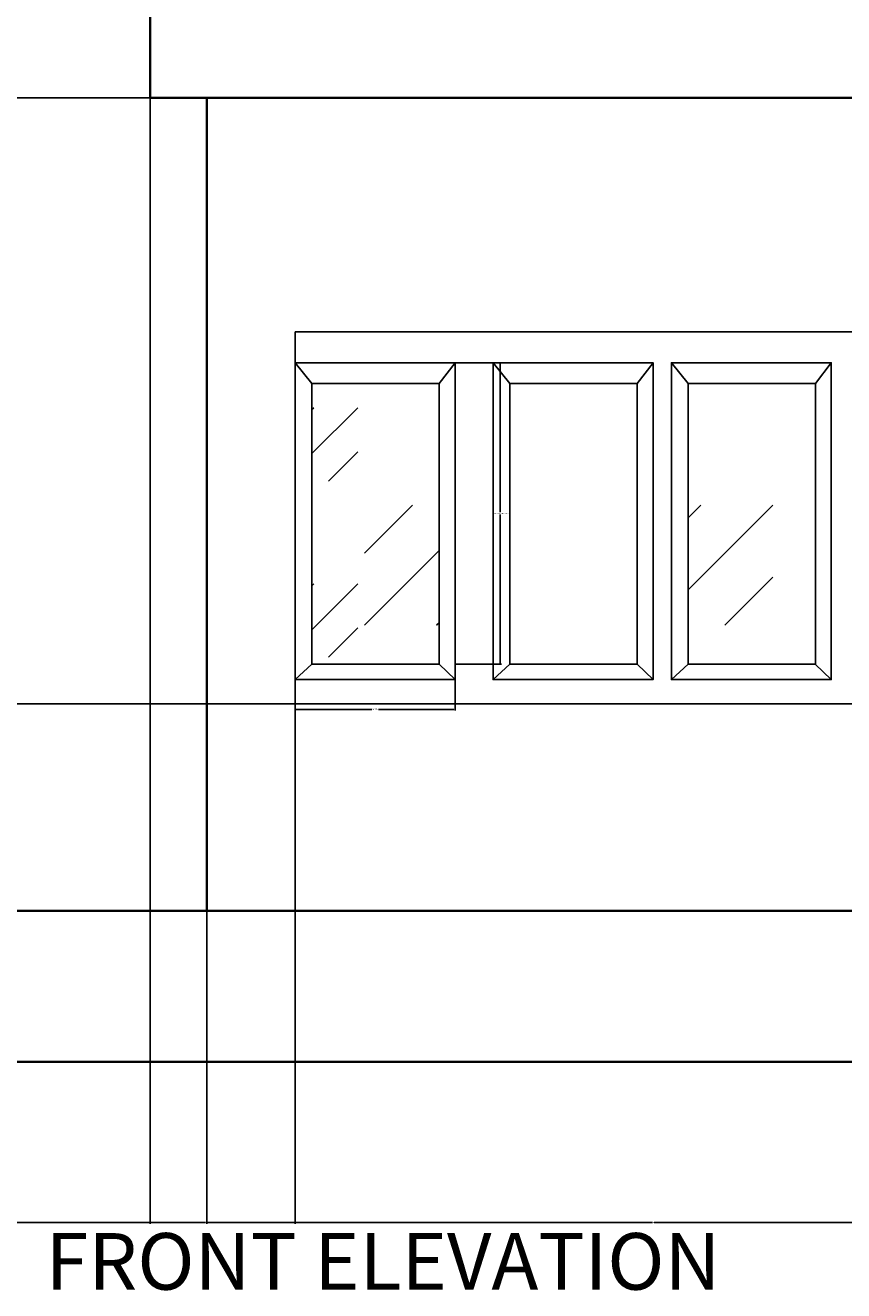
# Model space of a CAD drawing. Units: inches. Extents: x 93 to 565, y 123 to 656.
# Tile 2 of 18: x 267 to 397, y 123 to 324. Entities that reach past the tile are written whole.
import ezdxf

# ---------------------------------------------------------------- set-up
doc = ezdxf.new("R2010")
doc.units = ezdxf.units.IN
doc.header["$MEASUREMENT"] = 0
for name, color, linetype, lineweight in [('A-ANNO-DIMS', 2, 'Continuous', 18), ('A-ANNO-TEXT', 7, 'Continuous', 25), ('A-ELEV', 7, 'Continuous', 35), ('A-GLAZ', 4, 'Continuous', 25)]:
    doc.layers.add(name, color=color, linetype=linetype, lineweight=lineweight)
doc.styles.get("Standard").update_dxf_attribs({"font": 'arial.ttf'})
doc.dimstyles.get("Standard").update_dxf_attribs({"dimtxt": 0.18, "dimasz": 0.18, "dimexe": 0.18, "dimexo": 0.0625, "dimgap": 0.09, "dimtad": 0, "dimtih": 1, "dimtoh": 1, "dimdec": 4, "dimzin": 0, "dimdsep": 46, "dimtxsty": 'Standard', "dimcen": 0.09, "dimadec": 0, "dimazin": 0, "dimtfac": 1, "dimtdec": 4, "dimtofl": 0, "dimtmove": 0, "dimatfit": 3, "dimfxl": 1, "dimtolj": 1, "dimtzin": 0, "dimarcsym": 0})

# ---------------------------------------------------------------- blocks, each defined once
blk = doc.blocks.new('WIN-CASEMENT-LARGE')
blk.add_lwpolyline([(2.67, 44.6), (0, 47.91), (25.42, 47.91), (22.89, 44.6)])
blk.add_lwpolyline([(2.67, 44.6), (22.89, 44.6), (22.89, 0), (2.67, 0)], close=True)
blk = doc.blocks.new('*D18')
at = {"layer": 'A-ANNO-DIMS', "color": 0, "lineweight": -2, "transparency": 16777216}
for p, q in [((335.22, 270.85), (342.53, 270.85)), ((342.35, 270.67), (342.35, 247.08)), ((342.35, 223.12), (342.35, 246.71)), ((335.22, 222.94), (342.53, 222.94))]:
    blk.add_line(p, q, dxfattribs=at)
at = {"layer": 'A-ANNO-DIMS', "color": 0, "transparency": 16777216}
for points in [[(342.32, 270.67), (342.38, 270.67), (342.35, 270.85)], [(342.32, 223.12), (342.38, 223.12), (342.35, 222.94)]]:
    blk.add_solid(points, dxfattribs=at)
at = {"layer": 'Defpoints', "color": 0, "transparency": 16777216}
for p in [(335.16, 270.85), (342.35, 270.85), (335.16, 222.94)]:
    blk.add_point(p, dxfattribs=at)
at = {"layer": 'A-ANNO-DIMS', "color": 0, "transparency": 16777216, "insert": (342.35, 246.89), "char_height": 0.18, "attachment_point": 5}
blk.add_mtext('\\A1;LARGE WINDOW 48 TYP.', dxfattribs=at)
blk = doc.blocks.new('*D19')
at = {"layer": 'A-ANNO-DIMS', "color": 0, "lineweight": -2, "transparency": 16777216}
for p, q in [((309.74, 222.88), (309.74, 215.57)), ((335.16, 222.88), (335.16, 215.57)), ((309.92, 215.75), (321.92, 215.75)), ((334.98, 215.75), (322.98, 215.75))]:
    blk.add_line(p, q, dxfattribs=at)
at = {"layer": 'A-ANNO-DIMS', "color": 0, "transparency": 16777216}
for points in [[(309.92, 215.78), (309.92, 215.72), (309.74, 215.75)], [(334.98, 215.78), (334.98, 215.72), (335.16, 215.75)]]:
    blk.add_solid(points, dxfattribs=at)
at = {"layer": 'Defpoints', "color": 0, "transparency": 16777216}
for p in [(309.74, 222.94), (335.16, 222.94), (335.16, 215.75)]:
    blk.add_point(p, dxfattribs=at)
at = {"layer": 'A-ANNO-DIMS', "color": 0, "transparency": 16777216, "insert": (322.45, 215.75), "char_height": 0.18, "attachment_point": 5}
blk.add_mtext('\\A1;25 TYP.', dxfattribs=at)
blk = doc.blocks.new('*D28')
at = {"layer": 'A-ANNO-DIMS', "color": 0, "lineweight": -2, "transparency": 16777216}
for p, q in [((210.54, 519.04), (210.54, 134)), ((295.69, 183.67), (295.69, 134)), ((210.72, 134.18), (252.72, 134.18)), ((295.51, 134.18), (253.51, 134.18))]:
    blk.add_line(p, q, dxfattribs=at)
at = {"layer": 'A-ANNO-DIMS', "color": 0, "transparency": 16777216}
for points in [[(210.72, 134.21), (210.72, 134.15), (210.54, 134.18)], [(295.51, 134.21), (295.51, 134.15), (295.69, 134.18)]]:
    blk.add_solid(points, dxfattribs=at)
at = {"layer": 'Defpoints', "color": 0, "transparency": 16777216}
for p in [(210.54, 519.1), (295.69, 183.73), (295.69, 134.18)]:
    blk.add_point(p, dxfattribs=at)
at = {"layer": 'A-ANNO-DIMS', "color": 0, "transparency": 16777216, "insert": (253.12, 134.18), "char_height": 0.18, "attachment_point": 5}
blk.add_mtext('\\A1;85.14', dxfattribs=at)
blk = doc.blocks.new('*D29')
at = {"layer": 'A-ANNO-DIMS', "color": 0, "lineweight": -2, "transparency": 16777216}
for p, q in [((437.19, 594.34), (437.19, 134)), ((295.69, 183.67), (295.69, 134)), ((295.87, 134.18), (366.05, 134.18)), ((437.01, 134.18), (366.82, 134.18))]:
    blk.add_line(p, q, dxfattribs=at)
at = {"layer": 'A-ANNO-DIMS', "color": 0, "transparency": 16777216}
for points in [[(295.87, 134.21), (295.87, 134.15), (295.69, 134.18)], [(437.01, 134.21), (437.01, 134.15), (437.19, 134.18)]]:
    blk.add_solid(points, dxfattribs=at)
at = {"layer": 'Defpoints', "color": 0, "transparency": 16777216}
for p in [(437.19, 594.4), (295.69, 183.73), (437.19, 134.18)]:
    blk.add_point(p, dxfattribs=at)
at = {"layer": 'A-ANNO-DIMS', "color": 0, "transparency": 16777216, "insert": (366.44, 134.18), "char_height": 0.18, "attachment_point": 5}
blk.add_mtext('\\A1;141.5', dxfattribs=at)
blk = doc.blocks.new('*D31')
at = {"layer": 'A-ANNO-DIMS', "color": 0, "lineweight": -2, "transparency": 16777216}
for p, q in [((417.87, 630.4), (564.81, 630.4)), ((564.63, 630.22), (564.63, 395.25)), ((564.63, 159.91), (564.63, 394.89)), ((119.14, 159.73), (564.81, 159.73))]:
    blk.add_line(p, q, dxfattribs=at)
at = {"layer": 'A-ANNO-DIMS', "color": 0, "transparency": 16777216}
for points in [[(564.6, 630.22), (564.66, 630.22), (564.63, 630.4)], [(564.6, 159.91), (564.66, 159.91), (564.63, 159.73)]]:
    blk.add_solid(points, dxfattribs=at)
at = {"layer": 'Defpoints', "color": 0, "transparency": 16777216}
for p in [(417.81, 630.4), (564.63, 630.4), (119.08, 159.73)]:
    blk.add_point(p, dxfattribs=at)
at = {"layer": 'A-ANNO-DIMS', "color": 0, "transparency": 16777216, "insert": (564.63, 395.07), "char_height": 0.18, "attachment_point": 5}
blk.add_mtext('\\A1;470.7', dxfattribs=at)
blk = doc.blocks.new('*D33')
at = {"layer": 'A-ANNO-DIMS', "color": 0, "lineweight": -2, "transparency": 16777216}
for p, q in [((286.62, 312.95), (93.35, 312.95)), ((93.53, 312.77), (93.53, 248.52)), ((93.53, 183.91), (93.53, 248.16)), ((119.02, 183.73), (93.35, 183.73))]:
    blk.add_line(p, q, dxfattribs=at)
at = {"layer": 'A-ANNO-DIMS', "color": 0, "transparency": 16777216}
for points in [[(93.5, 312.77), (93.56, 312.77), (93.53, 312.95)], [(93.5, 183.91), (93.56, 183.91), (93.53, 183.73)]]:
    blk.add_solid(points, dxfattribs=at)
at = {"layer": 'Defpoints', "color": 0, "transparency": 16777216}
for p in [(93.53, 312.95), (286.69, 312.95), (119.08, 183.73)]:
    blk.add_point(p, dxfattribs=at)
at = {"layer": 'A-ANNO-DIMS', "color": 0, "transparency": 16777216, "insert": (93.53, 248.34), "char_height": 0.18, "attachment_point": 5}
blk.add_mtext('\\A1;129.22', dxfattribs=at)
blk = doc.blocks.new('*D34')
at = {"layer": 'A-ANNO-DIMS', "color": 0, "lineweight": -2, "transparency": 16777216}
for p, q in [((286.62, 363.73), (93.35, 363.73)), ((93.53, 363.55), (93.53, 338.52)), ((93.53, 313.13), (93.53, 338.16)), ((286.62, 312.95), (93.35, 312.95))]:
    blk.add_line(p, q, dxfattribs=at)
at = {"layer": 'A-ANNO-DIMS', "color": 0, "transparency": 16777216}
for points in [[(93.5, 363.55), (93.56, 363.55), (93.53, 363.73)], [(93.5, 313.13), (93.56, 313.13), (93.53, 312.95)]]:
    blk.add_solid(points, dxfattribs=at)
at = {"layer": 'Defpoints', "color": 0, "transparency": 16777216}
for p in [(93.53, 363.73), (286.69, 363.73), (286.69, 312.95)]:
    blk.add_point(p, dxfattribs=at)
at = {"layer": 'A-ANNO-DIMS', "color": 0, "transparency": 16777216, "insert": (93.53, 338.34), "char_height": 0.18, "attachment_point": 5}
blk.add_mtext('\\A1;50.78', dxfattribs=at)
blk = doc.blocks.new('*D51')
at = {"layer": 'A-ANNO-DIMS', "color": 0, "lineweight": -2, "transparency": 16777216}
for p, q in [((286.69, 312.89), (286.69, 134)), ((295.69, 312.89), (295.69, 134)), ((286.87, 134.18), (291.04, 134.18)), ((295.51, 134.18), (291.34, 134.18))]:
    blk.add_line(p, q, dxfattribs=at)
at = {"layer": 'A-ANNO-DIMS', "color": 0, "transparency": 16777216}
for points in [[(286.87, 134.21), (286.87, 134.15), (286.69, 134.18)], [(295.51, 134.21), (295.51, 134.15), (295.69, 134.18)]]:
    blk.add_solid(points, dxfattribs=at)
at = {"layer": 'Defpoints', "color": 0, "transparency": 16777216}
for p in [(286.69, 312.95), (295.69, 312.95), (295.69, 134.18)]:
    blk.add_point(p, dxfattribs=at)
at = {"layer": 'A-ANNO-DIMS', "color": 0, "transparency": 16777216, "insert": (291.19, 134.18), "char_height": 0.18, "attachment_point": 5}
blk.add_mtext('\\A1;9', dxfattribs=at)
blk = doc.blocks.new('*D55')
at = {"layer": 'A-ANNO-DIMS', "color": 0, "lineweight": -2, "transparency": 16777216}
for p, q in [((309.74, 216.57), (309.74, 134)), ((295.69, 183.67), (295.69, 134)), ((295.87, 134.18), (302.26, 134.18)), ((309.56, 134.18), (303.17, 134.18))]:
    blk.add_line(p, q, dxfattribs=at)
at = {"layer": 'A-ANNO-DIMS', "color": 0, "transparency": 16777216}
for points in [[(295.87, 134.21), (295.87, 134.15), (295.69, 134.18)], [(309.56, 134.21), (309.56, 134.15), (309.74, 134.18)]]:
    blk.add_solid(points, dxfattribs=at)
at = {"layer": 'Defpoints', "color": 0, "transparency": 16777216}
for p in [(309.74, 216.63), (295.69, 183.73), (309.74, 134.18)]:
    blk.add_point(p, dxfattribs=at)
at = {"layer": 'A-ANNO-DIMS', "color": 0, "transparency": 16777216, "insert": (302.72, 134.18), "char_height": 0.18, "attachment_point": 5}
blk.add_mtext('\\A1;14.056', dxfattribs=at)
blk = doc.blocks.new('*D56')
at = {"layer": 'A-ANNO-DIMS', "color": 0, "lineweight": -2, "transparency": 16777216}
for p, q in [((309.74, 275.71), (309.74, 134)), ((424.3, 275.71), (424.3, 134)), ((309.92, 134.18), (366.57, 134.18)), ((424.12, 134.18), (367.48, 134.18))]:
    blk.add_line(p, q, dxfattribs=at)
at = {"layer": 'A-ANNO-DIMS', "color": 0, "transparency": 16777216}
for points in [[(309.92, 134.21), (309.92, 134.15), (309.74, 134.18)], [(424.12, 134.21), (424.12, 134.15), (424.3, 134.18)]]:
    blk.add_solid(points, dxfattribs=at)
at = {"layer": 'Defpoints', "color": 0, "transparency": 16777216}
for p in [(309.74, 275.77), (424.3, 275.77), (424.3, 134.18)]:
    blk.add_point(p, dxfattribs=at)
at = {"layer": 'A-ANNO-DIMS', "color": 0, "transparency": 16777216, "insert": (367.02, 134.18), "char_height": 0.18, "attachment_point": 5}
blk.add_mtext('\\A1;114.56', dxfattribs=at)
blk = doc.blocks.new('*D58')
at = {"layer": 'A-ANNO-DIMS', "color": 0, "lineweight": -2, "transparency": 16777216}
for p, q in [((309.68, 216.63), (93.35, 216.63)), ((93.53, 216.45), (93.53, 200.36)), ((93.53, 183.91), (93.53, 200)), ((295.62, 183.73), (93.35, 183.73))]:
    blk.add_line(p, q, dxfattribs=at)
at = {"layer": 'A-ANNO-DIMS', "color": 0, "transparency": 16777216}
for points in [[(93.5, 216.45), (93.56, 216.45), (93.53, 216.63)], [(93.5, 183.91), (93.56, 183.91), (93.53, 183.73)]]:
    blk.add_solid(points, dxfattribs=at)
at = {"layer": 'Defpoints', "color": 0, "transparency": 16777216}
for p in [(309.74, 216.63), (93.53, 183.73), (295.69, 183.73)]:
    blk.add_point(p, dxfattribs=at)
at = {"layer": 'A-ANNO-DIMS', "color": 0, "transparency": 16777216, "insert": (93.53, 200.18), "char_height": 0.18, "attachment_point": 5}
blk.add_mtext('\\A1;32.9', dxfattribs=at)
blk = doc.blocks.new('*D107')
at = {"layer": 'A-ANNO-DIMS', "color": 0, "lineweight": -2, "transparency": 16777216}
for p, q in [((210.54, 519.04), (210.54, 134)), ((295.69, 183.67), (295.69, 134)), ((210.72, 134.18), (252.65, 134.18)), ((295.51, 134.18), (253.58, 134.18))]:
    blk.add_line(p, q, dxfattribs=at)
at = {"layer": 'A-ANNO-DIMS', "color": 0, "transparency": 16777216}
for points in [[(210.72, 134.21), (210.72, 134.15), (210.54, 134.18)], [(295.51, 134.21), (295.51, 134.15), (295.69, 134.18)]]:
    blk.add_solid(points, dxfattribs=at)
at = {"layer": 'Defpoints', "color": 0, "transparency": 16777216}
for p in [(210.54, 519.1), (295.69, 183.73), (295.69, 134.18)]:
    blk.add_point(p, dxfattribs=at)
at = {"layer": 'A-ANNO-DIMS', "color": 0, "transparency": 16777216, "insert": (253.12, 134.18), "char_height": 0.18, "attachment_point": 5}
blk.add_mtext('\\A1;85.143', dxfattribs=at)
blk = doc.blocks.new('*D108')
at = {"layer": 'A-ANNO-DIMS', "color": 0, "lineweight": -2, "transparency": 16777216}
for p, q in [((437.19, 594.34), (437.19, 134)), ((295.69, 183.67), (295.69, 134)), ((295.87, 134.18), (365.93, 134.18)), ((437.01, 134.18), (366.95, 134.18))]:
    blk.add_line(p, q, dxfattribs=at)
at = {"layer": 'A-ANNO-DIMS', "color": 0, "transparency": 16777216}
for points in [[(295.87, 134.21), (295.87, 134.15), (295.69, 134.18)], [(437.01, 134.21), (437.01, 134.15), (437.19, 134.18)]]:
    blk.add_solid(points, dxfattribs=at)
at = {"layer": 'Defpoints', "color": 0, "transparency": 16777216}
for p in [(437.19, 594.4), (295.69, 183.73), (437.19, 134.18)]:
    blk.add_point(p, dxfattribs=at)
at = {"layer": 'A-ANNO-DIMS', "color": 0, "transparency": 16777216, "insert": (366.44, 134.18), "char_height": 0.18, "attachment_point": 5}
blk.add_mtext('\\A1;141.501', dxfattribs=at)
blk = doc.blocks.new('*D110')
at = {"layer": 'A-ANNO-DIMS', "color": 0, "lineweight": -2, "transparency": 16777216}
for p, q in [((417.87, 630.4), (564.81, 630.4)), ((564.63, 630.22), (564.63, 395.25)), ((564.63, 159.91), (564.63, 394.89)), ((119.14, 159.73), (564.81, 159.73))]:
    blk.add_line(p, q, dxfattribs=at)
at = {"layer": 'A-ANNO-DIMS', "color": 0, "transparency": 16777216}
for points in [[(564.6, 630.22), (564.66, 630.22), (564.63, 630.4)], [(564.6, 159.91), (564.66, 159.91), (564.63, 159.73)]]:
    blk.add_solid(points, dxfattribs=at)
at = {"layer": 'Defpoints', "color": 0, "transparency": 16777216}
for p in [(417.81, 630.4), (564.63, 630.4), (119.08, 159.73)]:
    blk.add_point(p, dxfattribs=at)
at = {"layer": 'A-ANNO-DIMS', "color": 0, "transparency": 16777216, "insert": (564.63, 395.07), "char_height": 0.18, "attachment_point": 5}
blk.add_mtext('\\A1;470.673', dxfattribs=at)
blk = doc.blocks.new('*D112')
at = {"layer": 'A-ANNO-DIMS', "color": 0, "lineweight": -2, "transparency": 16777216}
for p, q in [((286.62, 312.95), (93.35, 312.95)), ((93.53, 312.77), (93.53, 248.52)), ((93.53, 183.91), (93.53, 248.16)), ((119.02, 183.73), (93.35, 183.73))]:
    blk.add_line(p, q, dxfattribs=at)
at = {"layer": 'A-ANNO-DIMS', "color": 0, "transparency": 16777216}
for points in [[(93.5, 312.77), (93.56, 312.77), (93.53, 312.95)], [(93.5, 183.91), (93.56, 183.91), (93.53, 183.73)]]:
    blk.add_solid(points, dxfattribs=at)
at = {"layer": 'Defpoints', "color": 0, "transparency": 16777216}
for p in [(93.53, 312.95), (286.69, 312.95), (119.08, 183.73)]:
    blk.add_point(p, dxfattribs=at)
at = {"layer": 'A-ANNO-DIMS', "color": 0, "transparency": 16777216, "insert": (93.53, 248.34), "char_height": 0.18, "attachment_point": 5}
blk.add_mtext('\\A1;129.217', dxfattribs=at)
blk = doc.blocks.new('*D113')
at = {"layer": 'A-ANNO-DIMS', "color": 0, "lineweight": -2, "transparency": 16777216}
for p, q in [((286.62, 363.73), (93.35, 363.73)), ((93.53, 363.55), (93.53, 338.52)), ((93.53, 313.13), (93.53, 338.16)), ((286.62, 312.95), (93.35, 312.95))]:
    blk.add_line(p, q, dxfattribs=at)
at = {"layer": 'A-ANNO-DIMS', "color": 0, "transparency": 16777216}
for points in [[(93.5, 363.55), (93.56, 363.55), (93.53, 363.73)], [(93.5, 313.13), (93.56, 313.13), (93.53, 312.95)]]:
    blk.add_solid(points, dxfattribs=at)
at = {"layer": 'Defpoints', "color": 0, "transparency": 16777216}
for p in [(93.53, 363.73), (286.69, 363.73), (286.69, 312.95)]:
    blk.add_point(p, dxfattribs=at)
at = {"layer": 'A-ANNO-DIMS', "color": 0, "transparency": 16777216, "insert": (93.53, 338.34), "char_height": 0.18, "attachment_point": 5}
blk.add_mtext('\\A1;50.783', dxfattribs=at)
blk = doc.blocks.new('*D130')
at = {"layer": 'A-ANNO-DIMS', "color": 0, "lineweight": -2, "transparency": 16777216}
for p, q in [((286.69, 312.89), (286.69, 134)), ((295.69, 312.89), (295.69, 134)), ((286.87, 134.18), (290.79, 134.18)), ((295.51, 134.18), (291.58, 134.18))]:
    blk.add_line(p, q, dxfattribs=at)
at = {"layer": 'A-ANNO-DIMS', "color": 0, "transparency": 16777216}
for points in [[(286.87, 134.21), (286.87, 134.15), (286.69, 134.18)], [(295.51, 134.21), (295.51, 134.15), (295.69, 134.18)]]:
    blk.add_solid(points, dxfattribs=at)
at = {"layer": 'Defpoints', "color": 0, "transparency": 16777216}
for p in [(286.69, 312.95), (295.69, 312.95), (295.69, 134.18)]:
    blk.add_point(p, dxfattribs=at)
at = {"layer": 'A-ANNO-DIMS', "color": 0, "transparency": 16777216, "insert": (291.19, 134.18), "char_height": 0.18, "attachment_point": 5}
blk.add_mtext('\\A1;9.000', dxfattribs=at)
blk = doc.blocks.new('*D134')
at = {"layer": 'A-ANNO-DIMS', "color": 0, "lineweight": -2, "transparency": 16777216}
for p, q in [((309.74, 216.57), (309.74, 134)), ((295.69, 183.67), (295.69, 134)), ((295.87, 134.18), (302.26, 134.18)), ((309.56, 134.18), (303.17, 134.18))]:
    blk.add_line(p, q, dxfattribs=at)
at = {"layer": 'A-ANNO-DIMS', "color": 0, "transparency": 16777216}
for points in [[(295.87, 134.21), (295.87, 134.15), (295.69, 134.18)], [(309.56, 134.21), (309.56, 134.15), (309.74, 134.18)]]:
    blk.add_solid(points, dxfattribs=at)
at = {"layer": 'Defpoints', "color": 0, "transparency": 16777216}
for p in [(309.74, 216.63), (295.69, 183.73), (309.74, 134.18)]:
    blk.add_point(p, dxfattribs=at)
at = {"layer": 'A-ANNO-DIMS', "color": 0, "transparency": 16777216, "insert": (302.72, 134.18), "char_height": 0.18, "attachment_point": 5}
blk.add_mtext('\\A1;14.056', dxfattribs=at)
blk = doc.blocks.new('*D135')
at = {"layer": 'A-ANNO-DIMS', "color": 0, "lineweight": -2, "transparency": 16777216}
for p, q in [((309.74, 275.71), (309.74, 134)), ((424.3, 275.71), (424.3, 134)), ((309.92, 134.18), (366.5, 134.18)), ((424.12, 134.18), (367.55, 134.18))]:
    blk.add_line(p, q, dxfattribs=at)
at = {"layer": 'A-ANNO-DIMS', "color": 0, "transparency": 16777216}
for points in [[(309.92, 134.21), (309.92, 134.15), (309.74, 134.18)], [(424.12, 134.21), (424.12, 134.15), (424.3, 134.18)]]:
    blk.add_solid(points, dxfattribs=at)
at = {"layer": 'Defpoints', "color": 0, "transparency": 16777216}
for p in [(309.74, 275.77), (424.3, 275.77), (424.3, 134.18)]:
    blk.add_point(p, dxfattribs=at)
at = {"layer": 'A-ANNO-DIMS', "color": 0, "transparency": 16777216, "insert": (367.02, 134.18), "char_height": 0.18, "attachment_point": 5}
blk.add_mtext('\\A1;114.560', dxfattribs=at)
blk = doc.blocks.new('*D137')
at = {"layer": 'A-ANNO-DIMS', "color": 0, "lineweight": -2, "transparency": 16777216}
for p, q in [((309.68, 216.63), (93.35, 216.63)), ((93.53, 216.45), (93.53, 200.36)), ((93.53, 183.91), (93.53, 200)), ((295.62, 183.73), (93.35, 183.73))]:
    blk.add_line(p, q, dxfattribs=at)
at = {"layer": 'A-ANNO-DIMS', "color": 0, "transparency": 16777216}
for points in [[(93.5, 216.45), (93.56, 216.45), (93.53, 216.63)], [(93.5, 183.91), (93.56, 183.91), (93.53, 183.73)]]:
    blk.add_solid(points, dxfattribs=at)
at = {"layer": 'Defpoints', "color": 0, "transparency": 16777216}
for p in [(309.74, 216.63), (93.53, 183.73), (295.69, 183.73)]:
    blk.add_point(p, dxfattribs=at)
at = {"layer": 'A-ANNO-DIMS', "color": 0, "transparency": 16777216, "insert": (93.53, 200.18), "char_height": 0.18, "attachment_point": 5}
blk.add_mtext('\\A1;32.897', dxfattribs=at)

msp = doc.modelspace()

# ---------------------------------------------------------------- hatches: boundary and pattern name
at = {"layer": 'A-GLAZ'}
h = msp.add_hatch(dxfattribs=at)
h.set_pattern_fill('GOST_GLASS', color=256, scale=3.3)
h.set_pattern_definition([(45, (0, 0), (28.0014, 0), [16.5, -23.1]), (45, (7, 0), (28.0014, 0), [6.6, -33]), (45, (0, 7), (28.0014, 0), [6.6, -33])])
h.paths.add_polyline_path([(332.6288, 267.5414), (312.4161, 267.5414), (312.4161, 222.941), (332.6288, 222.941)])
h.paths.add_polyline_path([(370.0743, 415.3107), (357.167, 415.3107), (357.167, 386.8299), (370.0743, 386.8299)])
h.paths.add_polyline_path([(390.168, 415.3107), (377.2607, 415.3107), (377.2607, 386.8299), (390.168, 386.8299)])
h.paths.add_polyline_path([(408.2592, 415.3107), (395.3518, 415.3107), (395.3518, 386.8299), (408.2592, 386.8299)])
h.paths.add_polyline_path([(427.0129, 415.3107), (414.1056, 415.3107), (414.1056, 386.8299), (427.0129, 386.8299)])
h = msp.add_hatch(dxfattribs=at)
h.set_pattern_fill('GOST_GLASS', color=256, scale=5.4)
h.set_pattern_definition([(45, (0, 0), (45.8205, 0), [27, -37.8]), (45, (11.455, 0), (45.8205, 0), [10.8, -54]), (45, (0, 11.455), (45.8205, 0), [10.8, -54])])
h.paths.add_polyline_path([(236.4617, 274.9686), (216.0562, 274.9686), (216.0562, 220.3466), (236.4617, 220.3466)])
h.paths.add_polyline_path([(258.8673, 274.9686), (237.4617, 274.9686), (237.4617, 220.3466), (258.8673, 220.3466)])
h.paths.add_polyline_path([(332.6288, 267.5414), (312.4161, 267.5414), (312.4161, 222.941), (332.6288, 222.941)])
h.paths.add_polyline_path([(366.6285, 270.8489), (341.2098, 270.8489), (341.2098, 220.4891), (366.6285, 220.4891)])
h.paths.add_polyline_path([(343.8825, 222.941), (364.0951, 222.941), (364.0951, 267.5414), (343.8825, 267.5414)], flags=16)
h.paths.add_polyline_path([(392.4256, 267.5414), (372.2129, 267.5414), (372.2129, 222.941), (392.4256, 222.941)])
h.paths.add_polyline_path([(421.7937, 267.5414), (401.581, 267.5414), (401.581, 222.941), (421.7937, 222.941)])

# ---------------------------------------------------------------- linework, layer by layer
at = {"layer": 'A-ELEV'}
for p, q in [((286.6874, 327.7323), (286.6874, 312.9491)), ((286.6874, 312.9491), (539.0794, 312.9491)), ((295.6874, 312.9491), (295.6874, 183.7323)), ((539.0794, 183.7323), (119.0794, 183.7323)), ((119.0794, 159.7323), (539.0794, 159.7323))]:
    msp.add_line(p, q, dxfattribs=at)
at = {"layer": 'A-GLAZ'}
for p, q in [((335.1622, 220.4891), (309.7435, 220.4891)), ((366.6285, 220.4891), (341.2098, 220.4891)), ((394.959, 220.4891), (369.5402, 220.4891))]:
    msp.add_line(p, q, dxfattribs=at)
msp.add_lwpolyline([(309.7435, 275.7732), (424.3037, 275.7732), (424.3037, 216.6296), (309.7435, 216.6296)], close=True, dxfattribs=at)
for points in [[(312.4161, 222.941), (309.7435, 220.4891), (309.7435, 270.8489)], [(335.1622, 270.8489), (335.1622, 220.4891), (332.6288, 222.941)], [(343.8825, 222.941), (341.2098, 220.4891), (341.2098, 270.8489)], [(366.6285, 270.8489), (366.6285, 220.4891), (364.0951, 222.941)], [(372.2129, 222.941), (369.5402, 220.4891), (369.5402, 270.8489)], [(394.959, 270.8489), (394.959, 220.4891), (392.4256, 222.941)]]:
    msp.add_lwpolyline(points, dxfattribs=at)

# ---------------------------------------------------------------- block references
for p in [(309.743, 222.941), (341.2093, 222.941), (369.5398, 222.941)]:
    msp.add_blockref('WIN-CASEMENT-LARGE', p, dxfattribs=at)

# ---------------------------------------------------------------- texts
at = {"layer": 'A-ANNO-TEXT', "insert": (270.0796, 132.509), "char_height": 9, "attachment_point": 1}
msp.add_mtext_dynamic_manual_height_columns('FRONT ELEVATION', width=162.170131, gutter_width=1, heights=[0], dxfattribs=at)

# ---------------------------------------------------------------- dimensions: what is measured, and where the dimension line sits
at = {"layer": 'A-ANNO-DIMS'}
for base, p1, p2, override, picture, middle in [((564.6294, 630.4048), (119.0794, 159.7323), (417.8097, 630.4048), {"dimdec": 1, "dimlfac": 1, "dimrnd": 0, "dimzin": 0, "dimdsep": 46, "dimlunit": 2}, '*D31', (564.6294, 395.0685)), ((564.62936, 630.40478), (119.07936, 159.73225), (417.80971, 630.40477), {"dimdec": 3, "dimlfac": 1, "dimrnd": 0, "dimzin": 0, "dimdsep": 46, "dimlunit": 2}, '*D110', (564.62936, 395.06851)), ((93.5294, 363.7323), (286.6874, 312.9491), (286.6874, 363.7323), {"dimdec": 3, "dimlfac": 1, "dimrnd": 0, "dimzin": 0, "dimdsep": 46, "dimlunit": 2}, '*D113', (93.5294, 338.3407)), ((93.5294, 363.7323), (286.6874, 312.9491), (286.6874, 363.7323), {"dimdec": 2, "dimlfac": 1, "dimrnd": 0, "dimzin": 0, "dimdsep": 46, "dimlunit": 2}, '*D34', (93.5294, 338.3407)), ((93.5294, 312.9491), (119.0794, 183.7323), (286.6874, 312.9491), {"dimdec": 3, "dimlfac": 1, "dimrnd": 0, "dimzin": 0, "dimdsep": 46, "dimlunit": 2}, '*D112', (93.5294, 248.3407)), ((93.5294, 312.9491), (119.0794, 183.7323), (286.6874, 312.9491), {"dimdec": 2, "dimlfac": 1, "dimrnd": 0, "dimzin": 0, "dimdsep": 46, "dimlunit": 2}, '*D33', (93.5294, 248.3407)), ((93.5294, 183.7323), (309.7435, 216.6296), (295.6874, 183.7323), {"dimdec": 3, "dimlfac": 1, "dimrnd": 0, "dimzin": 0, "dimdsep": 46, "dimlunit": 2}, '*D137', (93.5294, 200.1809)), ((93.5294, 183.7323), (309.7435, 216.6296), (295.6874, 183.7323), {"dimdec": 1, "dimlfac": 1, "dimrnd": 0, "dimzin": 0, "dimdsep": 46, "dimlunit": 2}, '*D58', (93.5294, 200.1809))]:
    dim = msp.add_linear_dim(base=base, p1=p1, p2=p2, angle=90, dimstyle='Standard', override=override, dxfattribs=at)
    dim.commit()
    dim.dimension.update_dxf_attribs({"geometry": picture, "text_midpoint": middle})
for base, p1, p2, override, picture, middle in [((437.1885, 134.1823), (295.6874, 183.7323), (437.1885, 594.4048), {"dimdec": 1, "dimlfac": 1, "dimrnd": 0, "dimzin": 0, "dimdsep": 46, "dimlunit": 2}, '*D29', (366.438, 134.1823)), ((437.1885, 134.1823), (295.6874, 183.7323), (437.1885, 594.4048), {"dimdec": 3, "dimlfac": 1, "dimrnd": 0, "dimzin": 0, "dimdsep": 46, "dimlunit": 2}, '*D108', (366.438, 134.1823)), ((295.6874, 134.1823), (210.5443, 519.0999), (295.6874, 183.7323), {"dimdec": 2, "dimlfac": 1, "dimrnd": 0, "dimzin": 0, "dimdsep": 46, "dimlunit": 2}, '*D28', (253.1158, 134.1823)), ((295.6874, 134.1823), (210.5443, 519.0999), (295.6874, 183.7323), {"dimdec": 3, "dimlfac": 1, "dimrnd": 0, "dimzin": 0, "dimdsep": 46, "dimlunit": 2}, '*D107', (253.1158, 134.1823)), ((295.6874, 134.1823), (286.6874, 312.9491), (295.6874, 312.9491), {"dimdec": 0, "dimlfac": 1, "dimrnd": 0, "dimzin": 0, "dimdsep": 46, "dimlunit": 2}, '*D51', (291.1874, 134.1823)), ((295.6874, 134.1823), (286.6874, 312.9491), (295.6874, 312.9491), {"dimdec": 3, "dimlfac": 1, "dimrnd": 0, "dimzin": 0, "dimdsep": 46, "dimlunit": 2}, '*D130', (291.1874, 134.1823)), ((424.3037, 134.1823), (309.7435, 275.7732), (424.3037, 275.7732), {"dimdec": 2, "dimlfac": 1, "dimrnd": 0, "dimzin": 0, "dimdsep": 46, "dimlunit": 2}, '*D56', (367.0236, 134.1823)), ((424.3037, 134.1823), (309.7435, 275.7732), (424.3037, 275.7732), {"dimdec": 3, "dimlfac": 1, "dimrnd": 0, "dimzin": 0, "dimdsep": 46, "dimlunit": 2}, '*D135', (367.0236, 134.1823)), ((309.7435, 134.1823), (295.6874, 183.7323), (309.7435, 216.6296), {"dimdec": 3, "dimlfac": 1, "dimrnd": 0, "dimzin": 0, "dimdsep": 46, "dimlunit": 2}, '*D55', (302.7154, 134.1823)), ((309.7435, 134.1823), (295.6874, 183.7323), (309.7435, 216.6296), {"dimdec": 3, "dimlfac": 1, "dimrnd": 0, "dimzin": 0, "dimdsep": 46, "dimlunit": 2}, '*D134', (302.7154, 134.1823))]:
    dim = msp.add_linear_dim(base=base, p1=p1, p2=p2, dimstyle='Standard', override=override, dxfattribs=at)
    dim.commit()
    dim.dimension.update_dxf_attribs({"geometry": picture, "text_midpoint": middle})
dim = msp.add_linear_dim(base=(342.3484, 270.8489), p1=(335.1622, 222.941), p2=(335.1622, 270.8489), angle=90, text='LARGE WINDOW <> TYP.', dimstyle='Standard', override={"dimdec": 0, "dimrnd": 0, "dimzin": 0, "dimlunit": 2}, dxfattribs=at)
dim.commit()
dim.dimension.update_dxf_attribs({"geometry": '*D18', "text_midpoint": (342.3484, 246.8949)})
dim = msp.add_linear_dim(base=(335.1622, 215.7548), p1=(309.7435, 222.941), p2=(335.1622, 222.941), text='<> TYP.', dimstyle='Standard', override={"dimdec": 0, "dimrnd": 0, "dimzin": 0, "dimlunit": 2}, dxfattribs=at)
dim.commit()
dim.dimension.update_dxf_attribs({"geometry": '*D19', "text_midpoint": (322.4528, 215.7548)})

doc.saveas('drawing.dxf')
